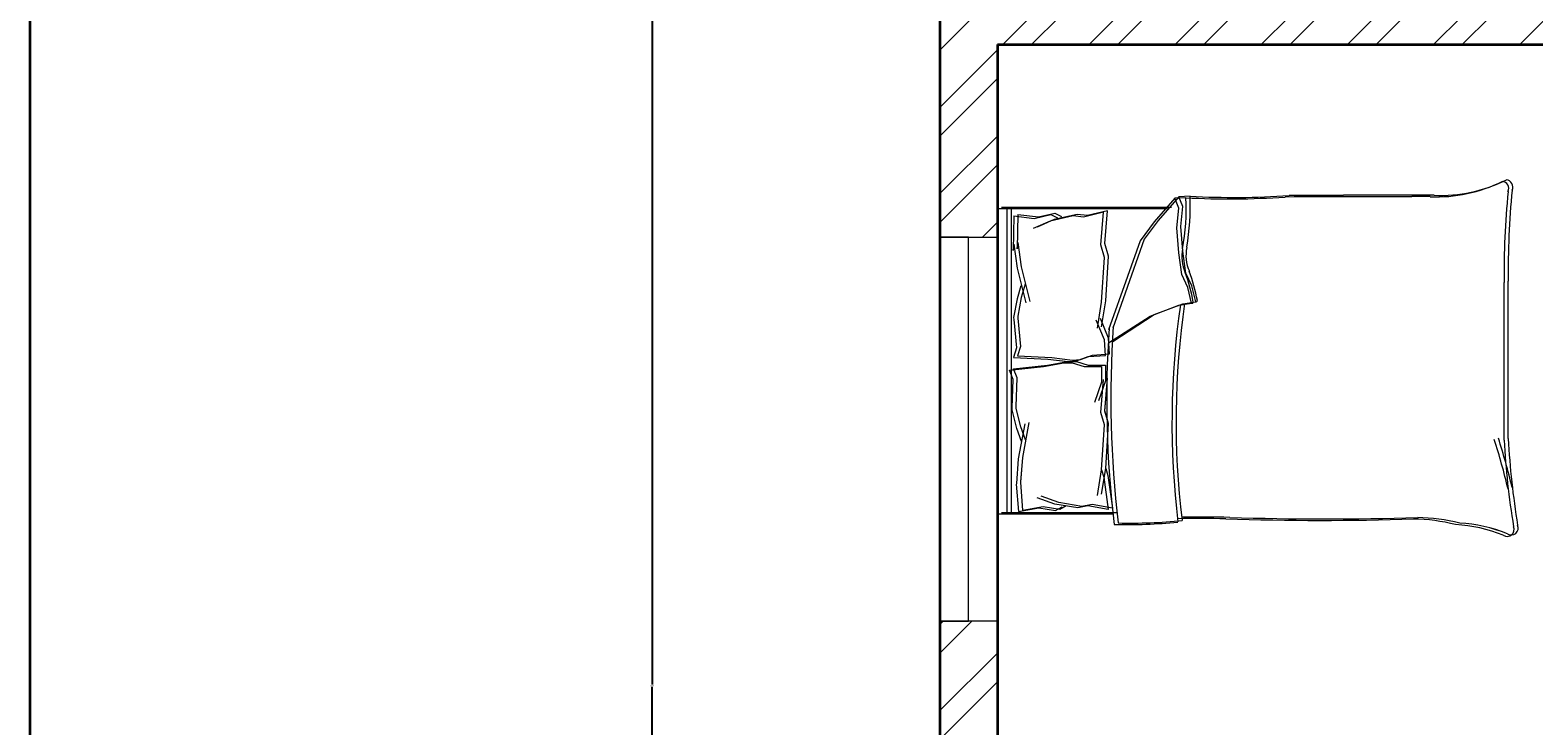
# Model space of a CAD drawing. Units: inches. Extents: x 2120 to 4013, y 1390 to 3019.
# Tile 27 of 59: x 2120 to 2356, y 1964 to 2073. Entities that reach past the tile are written whole.
import ezdxf

# ---------------------------------------------------------------- set-up
doc = ezdxf.new("R2010")
doc.units = ezdxf.units.IN
for name, color, linetype, lineweight in [('A-ANNO-DIMS', 2, 'Continuous', 18), ('A-ANNO-TTLB', 7, 'Continuous', 35), ('A-FURN', 8, 'Continuous', 13), ('A-GLAZ', 4, 'Continuous', 18), ('A-WALL', 7, 'Continuous', 35), ('A-WALL-PATT', 252, 'Continuous', 13)]:
    doc.layers.add(name, color=color, linetype=linetype, lineweight=lineweight)
doc.styles.get("Standard").update_dxf_attribs({"font": 'arial.ttf'})
doc.dimstyles.get("Standard").update_dxf_attribs({"dimtxt": 0.18, "dimasz": 0.18, "dimexe": 0.18, "dimexo": 0.0625, "dimgap": 0.09, "dimtad": 0, "dimtih": 1, "dimtoh": 1, "dimdec": 4, "dimzin": 0, "dimdsep": 46, "dimtxsty": 'Standard', "dimcen": 0.09, "dimadec": 0, "dimazin": 0, "dimtfac": 1, "dimtdec": 4, "dimtofl": 0, "dimtmove": 0, "dimatfit": 3, "dimfxl": 1, "dimtolj": 1, "dimtzin": 0, "dimarcsym": 0})

# ---------------------------------------------------------------- blocks, each defined once
blk = doc.blocks.new('BED-DOUBLE-PLAN')
for p, q in [((3.48, 63.34), (3.48, 81.45)), ((3.48, 81.45), (51.27, 81.45)), ((3.7, 62.7), (3.7, 80.81)), ((51.27, 81.45), (51.27, 54.84)), ((51.5, 80.81), (51.5, 54.2)), ((3.48, 79.91), (51.27, 79.91)), ((3.7, 79.27), (51.5, 79.27)), ((3.9, 78.11), (8.18, 78.44)), ((3.9, 78.13), (4.47, 74.95)), ((4.13, 77.47), (8.41, 77.8)), ((8.18, 78.44), (8.29, 78.42)), ((8.29, 78.42), (12.11, 78.13)), ((8.41, 77.8), (8.51, 77.78)), ((8.51, 77.78), (12.34, 77.49)), ((12.11, 78.13), (17.6, 77.12)), ((14.86, 77.7), (16.88, 78.42)), ((15.08, 77.06), (17.11, 77.78)), ((16.88, 78.42), (19.77, 79.14)), ((17.11, 77.78), (20, 78.5)), ((19.77, 79.14), (20.09, 79.14)), ((20, 78.5), (20.32, 78.5)), ((20.09, 79.14), (24.54, 79)), ((20.32, 78.5), (24.77, 78.36)), ((24.54, 79), (25.98, 79.58)), ((24.77, 78.36), (26.21, 78.94)), ((25.98, 79.58), (26.56, 74.23)), ((26.21, 78.94), (26.79, 73.59)), ((27.98, 78.95), (27.73, 73.58)), ((28.21, 78.32), (27.96, 72.94)), ((29.46, 78.47), (27.98, 78.95)), ((29.69, 77.83), (28.21, 78.32)), ((33.89, 78.89), (29.46, 78.47)), ((34.11, 78.25), (29.69, 77.83)), ((34.21, 78.91), (33.89, 78.89)), ((34.43, 78.27), (34.11, 78.25)), ((37.14, 78.37), (34.21, 78.91)), ((37.37, 77.73), (34.43, 78.27)), ((41.92, 78.38), (36.5, 77.02)), ((42.14, 77.74), (36.72, 76.38)), ((39.2, 77.77), (37.14, 78.37)), ((39.43, 77.13), (37.37, 77.73)), ((45.71, 78.9), (41.92, 78.38)), ((45.94, 78.26), (42.14, 77.74)), ((50.11, 78.89), (44.71, 78.99)), ((44.71, 78.99), (45.71, 78.9)), ((50.34, 78.25), (44.94, 78.35)), ((44.94, 78.35), (45.94, 78.26)), ((50.11, 78.89), (49.73, 75.68)), ((50.34, 78.25), (49.96, 75.04)), ((4.12, 77.49), (4.7, 74.31)), ((12.34, 77.49), (17.83, 76.48)), ((49.31, 73.19), (48.13, 75.87)), ((49.73, 75.68), (50.33, 73.11)), ((4.47, 74.95), (4.04, 72.35)), ((4.7, 74.31), (4.27, 71.71)), ((5.05, 72.49), (6.06, 75.24)), ((5.28, 71.85), (6.29, 74.6)), ((26.56, 74.23), (27.14, 71.05)), ((26.79, 73.59), (27.37, 70.41)), ((27.73, 73.58), (27.36, 70.37)), ((27.96, 72.94), (27.58, 69.73)), ((49.54, 72.55), (48.36, 75.23)), ((50.11, 69.62), (49.31, 73.19)), ((50.33, 73.11), (49.82, 72.06)), ((49.96, 75.04), (50.56, 72.47)), ((4.04, 72.35), (4.62, 71.33)), ((4.27, 71.71), (4.85, 70.7)), ((4.47, 68.88), (5.05, 72.49)), ((4.7, 68.24), (5.28, 71.85)), ((27.14, 71.05), (27.14, 69.74)), ((50.34, 68.98), (49.54, 72.55)), ((50.56, 72.47), (50.04, 71.42)), ((4.76, 67.29), (4.47, 68.88)), ((4.99, 66.65), (4.7, 68.24)), ((27.14, 69.74), (26.56, 67.86)), ((27.37, 69.1), (26.79, 67.23)), ((27.36, 70.37), (27.44, 69.07)), ((27.37, 70.41), (27.37, 69.1)), ((27.44, 69.07), (28.13, 67.23)), ((27.58, 69.73), (27.67, 68.43)), ((27.67, 68.43), (28.36, 66.59)), ((49.92, 68.01), (50.11, 69.62)), ((50.15, 67.37), (50.34, 68.98)), ((4.19, 64.11), (4.76, 67.29)), ((4.41, 63.47), (4.99, 66.65)), ((24.1, 65.18), (20.96, 66.27)), ((26.56, 67.86), (26.56, 65.18)), ((26.79, 67.23), (26.79, 64.54)), ((28.13, 67.23), (28.3, 64.55)), ((28.36, 66.59), (28.53, 63.91)), ((30.75, 64.71), (33.82, 65.99)), ((50.7, 64.87), (49.92, 68.01)), ((50.93, 64.23), (50.15, 67.37)), ((9.28, 64.83), (4.19, 64.11)), ((9.51, 64.19), (4.41, 63.47)), ((6.38, 65.82), (10.42, 65.15)), ((6.61, 65.18), (10.64, 64.51)), ((10.42, 65.15), (9.28, 64.83)), ((10.64, 64.51), (9.51, 64.19)), ((10.42, 65.15), (17.43, 64.72)), ((10.64, 64.51), (17.65, 64.08)), ((17.43, 64.72), (19.39, 65.28)), ((17.65, 64.08), (19.61, 64.64)), ((19.39, 65.28), (24.52, 64.87)), ((19.61, 64.64), (24.75, 64.23)), ((24.33, 64.54), (21.19, 65.63)), ((26.56, 65.18), (24.1, 65.18)), ((26.79, 64.54), (24.33, 64.54)), ((28.3, 64.55), (30.75, 64.71)), ((28.53, 63.91), (30.98, 64.07)), ((30.26, 64.06), (34.45, 57.57)), ((30.98, 64.07), (34.05, 65.35)), ((40.65, 61.13), (32.31, 64.06)), ((32.57, 65.82), (36.6, 65.15)), ((32.79, 65.18), (36.83, 64.51)), ((36.6, 65.15), (43.61, 64.72)), ((36.83, 64.51), (43.84, 64.08)), ((43.61, 64.72), (45.57, 65.28)), ((43.84, 64.08), (45.8, 64.64)), ((45.57, 65.28), (50.7, 64.87)), ((45.8, 64.64), (50.93, 64.23)), ((30.49, 63.42), (34.68, 56.93)), ((40.87, 60.49), (32.54, 63.42)), ((46.22, 59.12), (40.65, 61.13)), ((46.45, 58.48), (40.87, 60.49)), ((49.16, 56.95), (46.22, 59.12)), ((34.45, 57.57), (36.15, 53.08)), ((34.68, 56.93), (36.38, 52.44)), ((49.39, 56.31), (46.45, 58.48)), ((52.87, 53.7), (49.16, 56.95)), ((53.1, 53.06), (49.39, 56.31)), ((36.15, 53.08), (36.46, 51.07)), ((36.38, 52.44), (36.69, 50.43)), ((38.94, 51.69), (40.96, 52.62)), ((39.17, 51.05), (41.18, 51.98)), ((40.96, 52.62), (44.36, 53.08)), ((41.18, 51.98), (44.59, 52.44)), ((44.36, 53.08), (48.23, 53.39)), ((44.59, 52.44), (48.46, 52.75)), ((48.23, 53.39), (51.33, 53.08)), ((48.46, 52.75), (51.56, 52.44)), ((51.33, 53.08), (52.87, 53.7)), ((51.56, 52.44), (53.1, 53.06)), ((52.95, 51.96), (52.87, 53.7, 3.87)), ((53.18, 51.32), (53.1, 53.06, 3.87)), ((36.46, 51.07), (38.94, 51.69)), ((36.69, 50.43), (39.17, 51.05)), ((15.06, 2.2), (39.68, 2.2)), ((15.29, 1.56), (39.91, 1.56))]:
    blk.add_line(p, q)
for centre, radius, start, end in [((21.36, -100.61), 164.97, 86.0865, 96.7821), ((21.59, -101.25), 164.97, 86.0865, 96.7821), ((85.16, 61.35), 83.31, 178.7218, 185.604), ((85.39, 60.71), 83.31, 178.7218, 185.604), ((17.76, -74.87), 129.02, 81.7845, 96.9006), ((17.99, -75.51), 129.02, 81.7845, 96.9006), ((-167.31, 50.27), 170.11, 358.4762, 1.0082), ((-167.08, 49.63), 170.11, 358.4762, 1.0082), ((31.16, 79.96), 29.65, 280.6617, 289.8806), ((43.74, 46.38), 6.22, 78.6608, 113.7384), ((43.97, 45.74), 6.22, 78.6608, 113.7384), ((51.33, 88.1), 36.18, 259.8763, 272.5657), ((51.56, 87.46), 36.18, 259.8763, 272.5657), ((182.27, 45.13), 129.5, 176.9791, 183.8365), ((36.64, 51.01), 0.185, 160.2464, 271.1377), ((36.87, 50.37), 0.185, 160.2464, 271.1377), ((31.38, 79.32), 29.65, 280.6617, 289.8806), ((182.5, 44.49), 129.5, 176.9791, 183.8365), ((484.82, 30.83), 482.31, 178.2277, 181.7185), ((485.05, 30.19), 482.31, 178.2277, 181.7185), ((-4508.74, 13.62), 4561.86, 0.00217, 0.28689), ((-4508.51, 12.99), 4561.86, 0.00217, 0.28689), ((-26.9, 16.93), 29.63, 346.0648, 358.9113), ((-26.67, 16.29), 29.63, 346.0648, 358.9113), ((76.16, 12.78), 23.07, 177.4714, 206.4681), ((76.39, 12.14), 23.07, 177.4714, 206.4681), ((-21.66, 11.17), 23.56, 337.9751, 356.652), ((-21.43, 10.53), 23.56, 337.9751, 356.652), ((-17.22, 105.16), 106.46, 283.3832, 287.7053), ((-16.99, 104.52), 106.46, 283.3832, 287.7053), ((54.41, 2.58), 1.1, 242.6588, 356.02), ((1.09, 1.73), 1.09, 146.1736, 293.4781), ((1.32, 1.09), 1.09, 146.1736, 293.4781), ((21.43, -119.39), 121.76, 92.9958, 99.4091), ((21.66, -120.03), 121.76, 92.9958, 99.4091), ((41.15, -130.83), 133.04, 84.4998, 90.6351), ((41.38, -131.47), 133.04, 84.4998, 90.6351), ((54.64, 1.94), 1.1, 242.6588, 356.02)]:
    blk.add_arc(centre, radius, start, end)
blk = doc.blocks.new('WIN-PLAN-60IN-02')
for p, q in [((0, 0), (0, 9)), ((0, 9), (0, 4.5)), ((60, 4.5), (60, 9)), ((60, 9), (60, 0)), ((0, 4.5), (60, 4.5))]:
    blk.add_line(p, q)
blk = doc.blocks.new('*D214')
at = {"layer": 'A-ANNO-DIMS', "color": 0, "lineweight": -2, "transparency": 16777216}
for p, q in [((2271.67, 2075.03), (2217.55, 2075.03)), ((2217.73, 2074.85), (2217.73, 1970.46)), ((2217.73, 1865.71), (2217.73, 1970.1)), ((2271.67, 1865.53), (2217.55, 1865.53))]:
    blk.add_line(p, q, dxfattribs=at)
at = {"layer": 'A-ANNO-DIMS', "color": 0, "transparency": 16777216}
for points in [[(2217.7, 2074.85), (2217.76, 2074.85), (2217.73, 2075.03)], [(2217.7, 1865.71), (2217.76, 1865.71), (2217.73, 1865.53)]]:
    blk.add_solid(points, dxfattribs=at)
at = {"layer": 'Defpoints', "color": 0, "transparency": 16777216}
for p in [(2217.73, 2075.03), (2271.73, 2075.03), (2271.73, 1865.53)]:
    blk.add_point(p, dxfattribs=at)
at = {"layer": 'A-ANNO-DIMS', "color": 0, "transparency": 16777216, "insert": (2217.73, 1970.28), "char_height": 0.18, "attachment_point": 5}
blk.add_mtext('\\A1;209.5', dxfattribs=at)

msp = doc.modelspace()

# ---------------------------------------------------------------- hatches: boundary and pattern name
at = {"layer": 'A-WALL-PATT'}
h = msp.add_hatch(dxfattribs=at)
h.set_pattern_fill('ANSI32', color=256)
h.paths.add_polyline_path([(2271.7331, 1980.389), (2262.7331, 1980.389), (2262.7331, 1912.8434), (2267.2331, 1912.8434), (2271.7331, 1912.8434), (2271.7331, 1922.531), (2351.2331, 1922.531), (2351.2331, 1901.4728), (2355.7331, 1901.4728), (2355.7331, 1922.531), (2357.9815, 1922.531), (2357.9815, 1926.5306), (2271.7331, 1926.5306)])
h.paths.add_polyline_path([(2589.2331, 1949.1622), (2584.7331, 1949.1622), (2580.2331, 1949.1622), (2580.2331, 1874.5306), (2355.7331, 1874.5306), (2355.7331, 1880.1922), (2351.2331, 1880.1922), (2351.2331, 1874.5306), (2271.7331, 1874.5306), (2271.7331, 1888.8431), (2262.7331, 1888.8431), (2262.7331, 1842.2909), (2267.2331, 1842.2909), (2271.7331, 1842.2909), (2271.7331, 1865.531), (2415.7331, 1865.531), (2415.7331, 1779.7286), (2420.2331, 1779.7286), (2420.2331, 1865.531), (2589.2331, 1865.531)])
h.paths.add_polyline_path([(2271.7331, 1782.2906), (2262.7331, 1782.2906), (2262.7331, 1711.4639), (2267.2331, 1711.4639), (2271.7331, 1711.4639), (2271.7331, 1738.031), (2420.2331, 1738.031), (2420.2331, 1742.531), (2420.2331, 1747.3376), (2417.9831, 1747.3376), (2415.7331, 1747.3376), (2415.7331, 1742.5306), (2271.7331, 1742.5306)])
h.paths.add_polyline_path([(2271.7331, 1627.031), (2362.3957, 1627.031), (2362.3957, 1629.281), (2362.3957, 1631.5306), (2271.7331, 1631.5306), (2271.7331, 1675.4636), (2262.7331, 1675.4636), (2262.7331, 1581.531), (2405.3032, 1581.531), (2405.3032, 1586.031), (2405.3032, 1590.5306), (2396.2331, 1590.5306), (2396.2331, 1691.4513), (2418.7206, 1691.4513), (2418.7206, 1695.951), (2396.2331, 1695.951), (2391.7331, 1695.951), (2391.7331, 1631.5306), (2386.7425, 1631.5306), (2386.7425, 1629.2806), (2386.7425, 1627.031), (2391.7331, 1627.031), (2391.7331, 1586.1709), (2271.7331, 1586.1709)])
h.paths.add_polyline_path([(2459.6703, 1590.5306), (2429.3032, 1590.5306), (2429.3032, 1581.531), (2459.6703, 1581.531), (2459.6703, 1586.031)])
h.paths.add_polyline_path([(2501.2331, 1590.531), (2501.2331, 1665.0195), (2498.9831, 1665.0195), (2496.7331, 1665.0195), (2496.7331, 1590.5306), (2483.8201, 1590.5306), (2483.8201, 1590.1579), (2483.6704, 1590.1579), (2483.6704, 1581.531), (2505.0196, 1581.531), (2505.0196, 1583.781), (2505.0196, 1586.0306), (2501.2331, 1586.0306)])
h.paths.add_polyline_path([(2544.1361, 1583.781), (2544.1361, 1586.0306), (2527.1368, 1586.0306), (2527.1368, 1583.7806), (2527.1368, 1581.531), (2544.1361, 1581.531)])
h.paths.add_polyline_path([(3822.6535, 2458.4402), (3874.9468, 2458.4402), (3874.9468, 2476.9866), (3822.6535, 2476.9866)], flags=9)
h.paths.add_polyline_path([(3834.6921, 2781.8174), (3935.9206, 2781.8174), (3935.9206, 2800.3638), (3834.6921, 2800.3638)], flags=9)
h.paths.add_polyline_path([(3832.2843, 2837.9683), (3884.5776, 2837.9683), (3884.5776, 2856.5146), (3832.2843, 2856.5146)], flags=9)
h.paths.add_polyline_path([(3830.9388, 2861.4782), (3956.8958, 2861.4782), (3956.8958, 2880.0245), (3830.9388, 2880.0245)], flags=9)
h.paths.add_polyline_path([(3870.6966, 2352.5752), (3887.9272, 2352.5752), (3887.9272, 2377.3037), (3870.6966, 2377.3037)], flags=9)
h.paths.add_polyline_path([(3289.2701, 2413.161), (3435.2223, 2413.161), (3435.2223, 2450.2538), (3289.2701, 2450.2538)], flags=9)
h.paths.add_polyline_path([(2487.6944, 2414.3601), (2637.8335, 2414.3601), (2637.8335, 2451.4528), (2487.6944, 2451.4528)], flags=9)
h.paths.add_polyline_path([(2567.3724, 1457.9199), (2815.296, 1457.9199), (2815.296, 1495.0127), (2567.3724, 1495.0127)], flags=9)
h.paths.add_polyline_path([(2655.3825, 2093.2363), (2685.9555, 2093.2363), (2685.9555, 2111.8937), (2655.3825, 2111.8937)], flags=9)
h.paths.add_polyline_path([(2543.9218, 1550.6671), (2587.8406, 1550.6671), (2587.8406, 1569.3244), (2543.9218, 1569.3244)], flags=9)
h.paths.add_polyline_path([(2905.1384, 1543.8113), (2949.0572, 1543.8113), (2949.0572, 1562.4686), (2905.1384, 1562.4686)], flags=9)
h.paths.add_polyline_path([(2736.4118, 1702.4736), (2784.2153, 1702.4736), (2784.2153, 1721.1309), (2736.4118, 1721.1309)], flags=9)
h.paths.add_polyline_path([(2912.8666, 1710.4168), (2951.707, 1710.4168), (2951.707, 1729.0741), (2912.8666, 1729.0741)], flags=9)
h.paths.add_polyline_path([(2923.5785, 1763.5038), (2959.7279, 1763.5038), (2959.7279, 1782.1611), (2923.5785, 1782.1611)], flags=9)
h.paths.add_polyline_path([(2925.2114, 1809.6137), (2967.1861, 1809.6137), (2967.1861, 1828.271), (2925.2114, 1828.271)], flags=9)
h.paths.add_polyline_path([(2996.2711, 1878.9003), (2996.2711, 1913.109), (2977.6138, 1913.109), (2977.6138, 1878.9003)], flags=9)
h.paths.add_polyline_path([(2883.0859, 1895.7192), (2927.1855, 1895.7192), (2927.1855, 1914.3766), (2883.0859, 1914.3766)], flags=9)
h.paths.add_polyline_path([(2787.3924, 1810.8013), (2841.0213, 1810.8013), (2841.0213, 1829.4587), (2787.3924, 1829.4587)], flags=9)
h.paths.add_polyline_path([(2775.6399, 2101.7395), (2829.2689, 2101.7395), (2829.2689, 2120.3968), (2775.6399, 2120.3968)], flags=9)
h.paths.add_polyline_path([(2913.0263, 2075.817), (2951.8667, 2075.817), (2951.8667, 2094.4744), (2913.0263, 2094.4744)], flags=9)
h.paths.add_polyline_path([(2929.966, 2133.3669), (2966.1154, 2133.3669), (2966.1154, 2152.0243), (2929.966, 2152.0243)], flags=9)
h.paths.add_polyline_path([(2932.7502, 2182.6088), (2968.8996, 2182.6088), (2968.8996, 2201.2662), (2932.7502, 2201.2662)], flags=9)
h.paths.add_polyline_path([(2996.0681, 2266.3173), (2996.0681, 2300.5261), (2977.4108, 2300.5261), (2977.4108, 2266.3173)], flags=9)
h.paths.add_polyline_path([(2885.1039, 2279.2186), (2929.2035, 2279.2186), (2929.2035, 2297.8759), (2885.1039, 2297.8759)], flags=9)
h.paths.add_polyline_path([(2735.7042, 2218.3197), (2783.5078, 2218.3197), (2783.5078, 2236.9771), (2735.7042, 2236.9771)], flags=9)
h.paths.add_polyline_path([(2635.6049, 2044.0085), (2648.9678, 2044.0085), (2648.9678, 2054.312), (2635.6049, 2054.312)], flags=9)
h.paths.add_polyline_path([(2714.0148, 1923.0473), (2727.3777, 1923.0473), (2727.3777, 1933.3508), (2714.0148, 1933.3508)], flags=9)
h.paths.add_polyline_path([(2709.0345, 1988.1628), (2722.3974, 1988.1628), (2722.3974, 1998.4663), (2709.0345, 1998.4663)], flags=9)
h.paths.add_polyline_path([(2592.8935, 1962.1763), (2606.2564, 1962.1763), (2606.2564, 1972.4799), (2592.8935, 1972.4799)], flags=9)
h.paths.add_polyline_path([(2618.3996, 1985.9724), (2644.1942, 1985.9724), (2644.1942, 1996.2759), (2618.3996, 1996.2759)], flags=9)
h.paths.add_polyline_path([(2601.279, 1920.5869), (2614.6419, 1920.5869), (2614.6419, 1930.8904), (2601.279, 1930.8904)], flags=9)
h.paths.add_polyline_path([(2692.3278, 1932.7645), (2704.5311, 1932.7645), (2704.5311, 1943.0681), (2692.3278, 1943.0681)], flags=9)
h.paths.add_polyline_path([(2311.122, 1672.7318), (2355.0408, 1672.7318), (2355.0408, 1691.3892), (2311.122, 1691.3892)], flags=25)
h.paths.add_polyline_path([(2456.2551, 1632.3198), (2492.4796, 1632.3198), (2492.4796, 1650.9772), (2456.2551, 1650.9772)], flags=9)
h.paths.add_polyline_path([(2401.0766, 1631.4793), (2437.301, 1631.4793), (2437.301, 1650.1367), (2401.0766, 1650.1367)], flags=9)
h.paths.add_polyline_path([(2546.7054, 1700.9235), (2594.509, 1700.9235), (2594.509, 1719.5809), (2546.7054, 1719.5809)], flags=9)
h.paths.add_polyline_path([(2445.4866, 1766.9937), (2497.5261, 1766.9937), (2497.5261, 1785.651), (2445.4866, 1785.651)], flags=9)
h.paths.add_polyline_path([(2287.9992, 1739.7675), (2326.8396, 1739.7675), (2326.8396, 1758.4248), (2287.9992, 1758.4248)], flags=24)
h.paths.add_polyline_path([(2458.5279, 1924.7607), (2510.5675, 1924.7607), (2510.5675, 1943.4181), (2458.5279, 1943.4181)], flags=25)
h.paths.add_polyline_path([(2309.2811, 1902.7642), (2345.4305, 1902.7642), (2345.4305, 1921.4215), (2309.2811, 1921.4215)], flags=25)
h.paths.add_polyline_path([(2490.7554, 2018.9392), (2530.7896, 2018.9392), (2530.7896, 2037.5965), (2490.7554, 2037.5965)], flags=9)
h.paths.add_polyline_path([(2402.143, 2024.7393), (2438.5414, 2024.7393), (2438.5414, 2043.3966), (2402.143, 2043.3966)], flags=9)
h.paths.add_polyline_path([(2287.856, 1931.7926), (2326.6964, 1931.7926), (2326.6964, 1950.4499), (2287.856, 1950.4499)], flags=25)
h.paths.add_polyline_path([(2281.7979, 2193.5771), (2320.6383, 2193.5771), (2320.6383, 2212.2344), (2281.7979, 2212.2344)], flags=9)
h.paths.add_polyline_path([(2484.0754, 2093.892), (2536.115, 2093.892), (2536.115, 2112.5494), (2484.0754, 2112.5494)], flags=9)
h.paths.add_polyline_path([(2624.7948, 2281.8639), (2624.7948, 2311.4137), (2606.1375, 2311.4137), (2606.1375, 2281.8639)], flags=9)
h.paths.add_polyline_path([(2507.5036, 2290.3639), (2541.934, 2290.3639), (2541.934, 2309.0212), (2507.5036, 2309.0212)], flags=9)
h.paths.add_polyline_path([(2423.1076, 2285.2202), (2459.332, 2285.2202), (2459.332, 2303.8776), (2423.1076, 2303.8776)], flags=9)
h.paths.add_polyline_path([(2374.5467, 2289.6272), (2410.7711, 2289.6272), (2410.7711, 2308.2846), (2374.5467, 2308.2846)], flags=9)
h.paths.add_polyline_path([(2277.4907, 2227.5651), (2316.3311, 2227.5651), (2316.3311, 2246.2224), (2277.4907, 2246.2224)], flags=9)
h.paths.add_polyline_path([(2655.3825, 2093.2367), (2685.9555, 2093.2367), (2685.9555, 2111.894), (2655.3825, 2111.894)], flags=9)
h.paths.add_polyline_path([(2543.9217, 1550.6674), (2587.8406, 1550.6674), (2587.8406, 1569.3247), (2543.9217, 1569.3247)], flags=9)
h.paths.add_polyline_path([(2905.1384, 1543.8116), (2949.0572, 1543.8116), (2949.0572, 1562.4689), (2905.1384, 1562.4689)], flags=9)
h.paths.add_polyline_path([(2736.4118, 1702.4739), (2784.2153, 1702.4739), (2784.2153, 1721.1312), (2736.4118, 1721.1312)], flags=9)
h.paths.add_polyline_path([(2912.8666, 1710.4171), (2951.707, 1710.4171), (2951.707, 1729.0744), (2912.8666, 1729.0744)], flags=9)
h.paths.add_polyline_path([(2923.5785, 1763.5041), (2959.7279, 1763.5041), (2959.7279, 1782.1614), (2923.5785, 1782.1614)], flags=9)
h.paths.add_polyline_path([(2925.2114, 1809.614), (2967.1861, 1809.614), (2967.1861, 1828.2713), (2925.2114, 1828.2713)], flags=9)
h.paths.add_polyline_path([(2996.2711, 1878.9006), (2996.2711, 1913.1094), (2977.6137, 1913.1094), (2977.6137, 1878.9006)], flags=9)
h.paths.add_polyline_path([(2883.0859, 1895.7195), (2927.1855, 1895.7195), (2927.1855, 1914.3769), (2883.0859, 1914.3769)], flags=9)
h.paths.add_polyline_path([(2787.3924, 1810.8016), (2841.0213, 1810.8016), (2841.0213, 1829.459), (2787.3924, 1829.459)], flags=9)
h.paths.add_polyline_path([(2775.6399, 2101.7398), (2829.2688, 2101.7398), (2829.2688, 2120.3971), (2775.6399, 2120.3971)], flags=9)
h.paths.add_polyline_path([(2913.0263, 2075.8173), (2951.8667, 2075.8173), (2951.8667, 2094.4747), (2913.0263, 2094.4747)], flags=9)
h.paths.add_polyline_path([(2929.966, 2133.3672), (2966.1154, 2133.3672), (2966.1154, 2152.0246), (2929.966, 2152.0246)], flags=9)
h.paths.add_polyline_path([(2932.7502, 2182.6091), (2968.8996, 2182.6091), (2968.8996, 2201.2665), (2932.7502, 2201.2665)], flags=9)
h.paths.add_polyline_path([(2996.0681, 2266.3176), (2996.0681, 2300.5264), (2977.4108, 2300.5264), (2977.4108, 2266.3176)], flags=9)
h.paths.add_polyline_path([(2885.1039, 2279.2189), (2929.2035, 2279.2189), (2929.2035, 2297.8762), (2885.1039, 2297.8762)], flags=9)
h.paths.add_polyline_path([(2735.7042, 2218.32), (2783.5078, 2218.32), (2783.5078, 2236.9774), (2735.7042, 2236.9774)], flags=9)
h.paths.add_polyline_path([(2635.6048, 2044.0088), (2648.9677, 2044.0088), (2648.9677, 2054.3123), (2635.6048, 2054.3123)], flags=9)
h.paths.add_polyline_path([(2714.0148, 1923.0476), (2727.3777, 1923.0476), (2727.3777, 1933.3511), (2714.0148, 1933.3511)], flags=9)
h.paths.add_polyline_path([(2709.0345, 1988.1631), (2722.3974, 1988.1631), (2722.3974, 1998.4666), (2709.0345, 1998.4666)], flags=9)
h.paths.add_polyline_path([(2592.8935, 1962.1766), (2606.2564, 1962.1766), (2606.2564, 1972.4802), (2592.8935, 1972.4802)], flags=9)
h.paths.add_polyline_path([(2618.3995, 1985.9727), (2644.1942, 1985.9727), (2644.1942, 1996.2762), (2618.3995, 1996.2762)], flags=9)
h.paths.add_polyline_path([(2601.279, 1920.5872), (2614.6419, 1920.5872), (2614.6419, 1930.8908), (2601.279, 1930.8908)], flags=9)
h.paths.add_polyline_path([(2692.3278, 1932.7648), (2704.5311, 1932.7648), (2704.5311, 1943.0684), (2692.3278, 1943.0684)], flags=9)
h.paths.add_polyline_path([(2311.122, 1672.7321), (2355.0408, 1672.7321), (2355.0408, 1691.3895), (2311.122, 1691.3895)], flags=25)
h.paths.add_polyline_path([(2456.2551, 1632.3201), (2492.4795, 1632.3201), (2492.4795, 1650.9775), (2456.2551, 1650.9775)], flags=9)
h.paths.add_polyline_path([(2401.0766, 1631.4796), (2437.301, 1631.4796), (2437.301, 1650.137), (2401.0766, 1650.137)], flags=9)
h.paths.add_polyline_path([(2546.7054, 1700.9238), (2594.509, 1700.9238), (2594.509, 1719.5812), (2546.7054, 1719.5812)], flags=9)
h.paths.add_polyline_path([(2445.4866, 1766.994), (2497.5261, 1766.994), (2497.5261, 1785.6513), (2445.4866, 1785.6513)], flags=9)
h.paths.add_polyline_path([(2287.9992, 1739.7678), (2326.8396, 1739.7678), (2326.8396, 1758.4251), (2287.9992, 1758.4251)], flags=24)
h.paths.add_polyline_path([(2458.5279, 1924.7611), (2510.5675, 1924.7611), (2510.5675, 1943.4184), (2458.5279, 1943.4184)], flags=25)
h.paths.add_polyline_path([(2309.2811, 1902.7645), (2345.4305, 1902.7645), (2345.4305, 1921.4218), (2309.2811, 1921.4218)], flags=25)
h.paths.add_polyline_path([(2490.7554, 2018.9395), (2530.7895, 2018.9395), (2530.7895, 2037.5968), (2490.7554, 2037.5968)], flags=9)
h.paths.add_polyline_path([(2402.143, 2024.7396), (2438.5413, 2024.7396), (2438.5413, 2043.3969), (2402.143, 2043.3969)], flags=9)
h.paths.add_polyline_path([(2287.856, 1931.7929), (2326.6964, 1931.7929), (2326.6964, 1950.4502), (2287.856, 1950.4502)], flags=25)
h.paths.add_polyline_path([(2281.7979, 2193.5774), (2320.6383, 2193.5774), (2320.6383, 2212.2347), (2281.7979, 2212.2347)], flags=9)
h.paths.add_polyline_path([(2484.0754, 2093.8924), (2536.115, 2093.8924), (2536.115, 2112.5497), (2484.0754, 2112.5497)], flags=9)
h.paths.add_polyline_path([(2624.7948, 2281.8642), (2624.7948, 2311.414), (2606.1374, 2311.414), (2606.1374, 2281.8642)], flags=9)
h.paths.add_polyline_path([(2507.5035, 2290.3642), (2541.934, 2290.3642), (2541.934, 2309.0215), (2507.5035, 2309.0215)], flags=9)
h.paths.add_polyline_path([(2423.1075, 2285.2205), (2459.332, 2285.2205), (2459.332, 2303.8779), (2423.1075, 2303.8779)], flags=9)
h.paths.add_polyline_path([(2374.5467, 2289.6275), (2410.7711, 2289.6275), (2410.7711, 2308.2849), (2374.5467, 2308.2849)], flags=9)
h.paths.add_polyline_path([(2277.4907, 2227.5654), (2316.3311, 2227.5654), (2316.3311, 2246.2227), (2277.4907, 2246.2227)], flags=9)
h = msp.add_hatch(dxfattribs=at)
h.set_pattern_fill('ANSI32', color=256)
h.paths.add_polyline_path([(2271.7331, 2122.6377), (2262.7331, 2122.6377), (2262.7331, 2040.3893), (2267.2331, 2040.3893), (2271.7331, 2040.3893), (2271.7331, 2044.8856), (2271.7331, 2070.531), (2391.7331, 2070.531), (2391.7331, 1926.5306), (2388.3993, 1926.5306), (2388.3993, 1922.531), (2395.7331, 1922.531), (2395.7331, 1992.531), (2400.4511, 1992.531), (2400.4511, 1997.0306), (2395.7331, 1997.0306), (2395.7331, 2070.531), (2443.7331, 2070.531), (2443.7331, 2046.1368), (2448.2331, 2046.1368), (2448.2331, 2070.531), (2580.2331, 2070.531), (2580.2331, 1997.0306), (2492.9076, 1997.0306), (2492.9076, 1992.531), (2580.2331, 1992.531), (2580.2331, 1983.9368), (2589.2331, 1983.9368), (2589.2331, 2070.531), (2589.2331, 2075.0306), (2396.2331, 2075.0306), (2396.2331, 2184.3565), (2393.9831, 2184.3565), (2391.7331, 2184.3565), (2391.7331, 2075.0306), (2271.7331, 2075.0306)])
h.paths.add_polyline_path([(2724.7331, 2138.0306), (2628.7331, 2138.0306), (2628.7331, 2070.5306), (2628.7331, 2067.0987), (2633.2331, 2067.0987), (2637.7331, 2067.0987), (2637.7331, 2070.531), (2657.3413, 2070.531), (2657.3413, 2079.5306), (2637.7331, 2079.5306), (2637.7331, 2129.031), (2715.7331, 2129.031), (2715.7331, 2079.5306), (2698.0378, 2079.5306), (2698.0378, 2070.531), (2715.7331, 2070.531), (2715.7331, 2012.1531), (2720.2331, 2012.1531), (2724.7331, 2012.1531)])
h.paths.add_polyline_path([(2724.7331, 2213.031), (2831.3209, 2213.031), (2831.3209, 2215.281), (2831.3209, 2217.5306), (2724.7331, 2217.5306), (2724.7331, 2343.531), (2751.8755, 2343.531), (2751.8755, 2352.5306), (2715.7331, 2352.5306), (2715.7331, 2138.031), (2724.7331, 2138.031)])
h.paths.add_polyline_path([(2902.53, 2352.5306), (2811.8755, 2352.5306), (2811.8755, 2343.531), (2867.2331, 2343.531), (2867.2331, 2217.5306), (2863.6364, 2217.5306), (2863.6364, 2213.031), (2871.7331, 2213.031), (2871.7331, 2217.531), (2871.7331, 2343.531), (2902.53, 2343.531)])
h.paths.add_polyline_path([(3009.7331, 2352.5306), (2938.53, 2352.5306), (2938.53, 2343.531), (2966.2331, 2343.531), (2966.2331, 2242.3281), (2968.4831, 2242.3281), (2970.7331, 2242.3281), (2970.7331, 2343.531), (3009.7331, 2343.531)])
h.paths.add_polyline_path([(3009.7331, 2217.5306), (2970.7331, 2217.5306), (2970.7331, 2220.5422), (2968.4831, 2220.5422), (2966.2331, 2220.5422), (2966.2331, 2217.5306), (2911.7752, 2217.5306), (2907.7331, 2217.5306), (2907.7331, 2213.0306), (2907.7331, 2194.9663), (2912.2331, 2194.9663), (2912.2331, 2213.031), (2970.7331, 2213.031), (3000.7331, 2213.031), (3000.7331, 2205.523), (3009.7331, 2205.523)])
h.paths.add_polyline_path([(3009.7331, 2181.5227), (3000.7331, 2181.5227), (3000.7331, 2165.0306), (2912.2331, 2165.0306), (2912.2331, 2170.8202), (2907.7331, 2170.8202), (2907.7331, 2165.0306), (2899.5169, 2165.0306), (2899.5169, 2162.7806), (2899.5169, 2160.531), (2907.7331, 2160.531), (2907.7331, 2137.3432), (2912.2331, 2137.3432), (2912.2331, 2160.531), (3000.7331, 2160.531), (3000.7331, 2150.4993), (3009.7331, 2150.4993)])
h.paths.add_polyline_path([(3009.7331, 2126.499), (3005.2331, 2126.499), (3000.7331, 2126.499), (3000.7331, 2112.5306), (2912.2331, 2112.5306), (2912.2331, 2115.6036), (2907.7331, 2115.6036), (2907.7331, 2108.031), (3000.7331, 2108.031), (3000.7331, 2084.7256), (3009.7331, 2084.7256)], flags=17)
h.paths.add_polyline_path([(3009.7331, 1971.531), (3009.7331, 2024.7253), (3000.7331, 2024.7253), (3000.7331, 2006.4153), (3000.7331, 1971.5306), (2864.2331, 1971.5306), (2864.2331, 2160.531), (2868.0522, 2160.531), (2868.0522, 2165.0306), (2859.7331, 2165.0306), (2859.7331, 1971.5306), (2724.7331, 1971.5306), (2724.7331, 1977.7012), (2715.7331, 1977.7012), (2715.7331, 1962.5306), (2715.7331, 1950.9035), (2720.2331, 1950.9035), (2724.7331, 1950.9035), (2724.7331, 1962.531), (2855.2331, 1962.531), (2859.7331, 1962.531), (2859.7331, 1835.031), (2864.2331, 1834.8158), (2864.2331, 1962.531), (2958.7331, 1962.531), (2958.7331, 1937.0925), (2963.2331, 1937.0925), (2963.2331, 1962.531), (3000.7331, 1962.531), (3009.7331, 1962.531)])
h.paths.add_polyline_path([(2724.7331, 1728.531), (2822.7164, 1728.531), (2822.7164, 1733.0306), (2724.7331, 1733.0306), (2724.7331, 1779.3416), (2715.7331, 1779.3416), (2715.7331, 1581.531), (2753.02, 1581.531), (2753.02, 1586.031), (2753.02, 1590.5306), (2724.7331, 1590.5306)])
h.paths.add_polyline_path([(2864.2331, 1590.531), (2864.2331, 1787.031), (2868.4075, 1787.031), (2868.4075, 1791.5306), (2859.7331, 1791.5306), (2859.7331, 1739.0306), (2859.7331, 1733.0306), (2854.3125, 1733.0306), (2854.3125, 1728.531), (2859.7331, 1728.531), (2859.7331, 1590.5306), (2813.02, 1590.5306), (2813.02, 1581.531), (2868.4123, 1581.531), (2868.4123, 1583.781), (2868.4123, 1586.0306), (2864.2331, 1586.0306)])
h.paths.add_polyline_path([(3009.7331, 1754.6619), (3000.7331, 1754.6619), (3000.7331, 1739.0306), (2912.2331, 1739.0306), (2912.2331, 1742.2257), (2907.7331, 1742.2257), (2907.7331, 1739.0306), (2907.7331, 1734.531), (3000.7331, 1734.531), (3000.7331, 1590.5306), (3000.7331, 1586.0306), (2971.3921, 1586.0306), (2971.3921, 1581.531), (3009.7331, 1581.531)])
h.paths.add_polyline_path([(2911.3921, 1583.781), (2911.3921, 1586.0306), (2891.2138, 1586.0306), (2891.2138, 1581.531), (2911.3921, 1581.531)])
h.paths.add_polyline_path([(3009.7331, 1799.8422), (3000.7331, 1799.8422), (3000.7331, 1791.5306), (2912.2331, 1791.5306), (2912.2331, 1796.3264), (2909.9831, 1796.3264), (2907.7331, 1796.3264), (2907.7331, 1791.5306), (2902.7033, 1791.5306), (2902.7033, 1787.031), (2907.7331, 1787.031), (2907.7331, 1761.1622), (2912.2331, 1761.1622), (2912.2331, 1787.031), (3000.7331, 1787.031), (3000.7331, 1778.6622), (3009.7331, 1778.6622)])
h.paths.add_polyline_path([(3009.7331, 1839.5306), (2963.2331, 1839.5306), (2963.2331, 1842.8629), (2960.9831, 1842.8629), (2958.7331, 1842.8629), (2958.7331, 1839.5306), (2907.7331, 1839.5306), (2907.7331, 1814.4599), (2912.2331, 1814.4599), (2912.2331, 1835.031), (3000.7331, 1835.031), (3000.7331, 1823.8425), (3009.7331, 1823.8425), (3009.7331, 1835.031)])
h.paths.add_polyline_path([(2963.2331, 1901.0922), (2960.9831, 1901.0922), (2958.7331, 1901.0922), (2958.7331, 1862.8843), (2963.2331, 1862.8843)], flags=17)
h.paths.add_polyline_path([(2724.7331, 1891.9826), (2724.7331, 1914.3416), (2715.7331, 1914.3416), (2715.7331, 1783.8416), (2637.7331, 1783.8416), (2637.7331, 1914.3416), (2628.7331, 1914.3416), (2624.7701, 1914.3416), (2624.7701, 1909.8416), (2624.7701, 1905.3419), (2628.7331, 1905.3419), (2628.7331, 1876.9915), (2628.7331, 1779.3419), (2637.7331, 1779.3419), (2715.7331, 1779.3419), (2724.7331, 1779.3419), (2724.7331, 1835.031)])
h.paths.add_polyline_path([(2637.7331, 1731.531), (2637.7331, 1779.3416), (2628.7331, 1779.3416), (2628.7331, 1731.5306), (2589.2331, 1731.5306), (2535.9814, 1731.5306), (2496.7331, 1731.5306), (2496.7331, 1725.6876), (2498.9831, 1725.6876), (2501.2331, 1725.6876), (2501.2331, 1727.031), (2628.7331, 1727.031), (2628.7331, 1680.4203), (2628.7331, 1590.5306), (2628.7331, 1586.0306), (2604.1361, 1586.0306), (2604.1361, 1581.531), (2637.7331, 1581.531), (2637.7331, 1590.531)])

# ---------------------------------------------------------------- linework, layer by layer
at = {"layer": 'A-ANNO-TTLB'}
msp.add_lwpolyline([(2120.4581, 3019.1237), (4012.9334, 3019.1237), (4012.9334, 1390.2222), (2120.4581, 1390.2222)], close=True, dxfattribs=at)
at = {"layer": 'A-WALL'}
for p, q in [((2262.7331, 2352.531), (2262.7331, 1581.531)), ((2262.7331, 2352.5306), (2262.7331, 1581.5306)), ((2271.7331, 2070.531), (2391.7331, 2070.531)), ((2271.7331, 2070.531), (2271.7331, 1926.531)), ((2271.7331, 2070.5306), (2391.7331, 2070.5306)), ((2271.7331, 2070.5306), (2271.7331, 1926.5306))]:
    msp.add_line(p, q, dxfattribs=at)

# ---------------------------------------------------------------- block references
at = {"layer": 'A-FURN'}
for p, rotation in [((2353.1794, 1993.6187), 89.99999999999996), ((2353.1794, 1993.6184), 89.99999999999999)]:
    msp.add_blockref('BED-DOUBLE-PLAN', p, dxfattribs=dict(at, rotation=rotation))
at = {"layer": 'A-GLAZ'}
for p, rotation in [((2271.7331, 1980.3893), 89.99999999999825), ((2271.7331, 1980.389), 89.99999999999895)]:
    msp.add_blockref('WIN-PLAN-60IN-02', p, dxfattribs=dict(at, rotation=rotation))

# ---------------------------------------------------------------- dimensions: what is measured, and where the dimension line sits
at = {"layer": 'A-ANNO-DIMS'}
dim = msp.add_linear_dim(base=(2217.7331, 2075.031), p1=(2271.7331, 1865.531), p2=(2271.7331, 2075.031), angle=90, dimstyle='Standard', override={"dimdec": 1, "dimlfac": 1, "dimrnd": 0, "dimzin": 0, "dimdsep": 46, "dimlunit": 2}, dxfattribs=at)
dim.commit()
dim.dimension.update_dxf_attribs({"geometry": '*D214', "text_midpoint": (2217.7331, 1970.281)})

doc.saveas('drawing.dxf')
